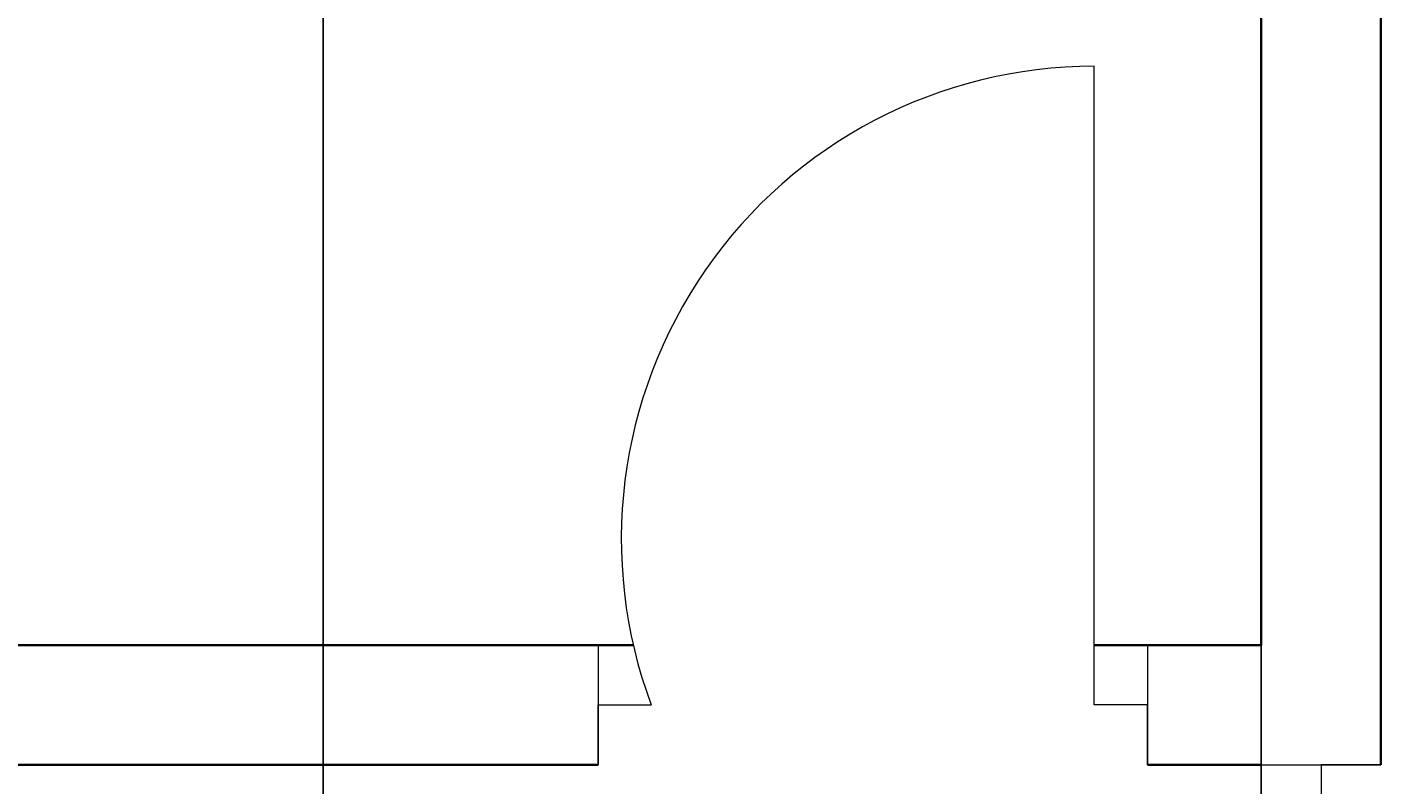
# Model space of a CAD drawing. Units: inches. Extents: x 1088 to 1703, y 668 to 1875.
# Tile 30 of 45: x 1539 to 1590, y 1539 to 1567. Entities that reach past the tile are written whole.
import ezdxf

# ---------------------------------------------------------------- set-up
doc = ezdxf.new("R2010")
doc.units = ezdxf.units.IN
for name, color, linetype, lineweight in [('A-ANNO-DIMS', 2, 'Continuous', 18), ('A-DOOR', 4, 'Continuous', 18), ('A-WALL', 7, 'Continuous', 35)]:
    doc.layers.add(name, color=color, linetype=linetype, lineweight=lineweight)
doc.styles.get("Standard").update_dxf_attribs({"font": 'arial.ttf'})
doc.dimstyles.get("Standard").update_dxf_attribs({"dimtxt": 0.18, "dimasz": 0.18, "dimexe": 0.18, "dimexo": 0.0625, "dimgap": 0.09, "dimtad": 0, "dimtih": 1, "dimtoh": 1, "dimdec": 4, "dimzin": 0, "dimdsep": 46, "dimtxsty": 'Standard', "dimcen": 0.09, "dimadec": 0, "dimazin": 0, "dimtfac": 1, "dimtdec": 4, "dimtofl": 0, "dimtmove": 0, "dimatfit": 3, "dimfxl": 1, "dimtolj": 1, "dimtzin": 0, "dimarcsym": 0})

# ---------------------------------------------------------------- blocks, each defined once
blk = doc.blocks.new('*D32')
at = {"layer": 'A-ANNO-DIMS', "color": 0, "lineweight": -2, "transparency": 16777216}
for p, q in [((1550.595, 1373.121), (1550.595, 1857.788)), ((1550.775, 1857.608), (1567.825, 1857.608)), ((1585.665, 1857.608), (1568.614, 1857.608)), ((1585.845, 1360.983), (1585.845, 1857.788))]:
    blk.add_line(p, q, dxfattribs=at)
at = {"layer": 'A-ANNO-DIMS', "color": 0, "transparency": 16777216}
for points in [[(1550.775, 1857.638), (1550.775, 1857.578), (1550.595, 1857.608)], [(1585.665, 1857.638), (1585.665, 1857.578), (1585.845, 1857.608)]]:
    blk.add_solid(points, dxfattribs=at)
at = {"layer": 'Defpoints', "color": 0, "transparency": 16777216}
for p in [(1585.845, 1857.608), (1550.595, 1373.058), (1585.845, 1360.921)]:
    blk.add_point(p, dxfattribs=at)
at = {"layer": 'A-ANNO-DIMS', "color": 0, "transparency": 16777216, "insert": (1568.22, 1857.608), "char_height": 0.18, "attachment_point": 5}
blk.add_mtext('\\A1;35.25', dxfattribs=at)

msp = doc.modelspace()

# ---------------------------------------------------------------- linework, layer by layer
at = {"layer": 'A-DOOR'}
for p, q in [((1579.571, 1541.808), (1579.571, 1565.808)), ((1560.928, 1544.058), (1560.928, 1539.558)), ((1581.571, 1544.058), (1581.571, 1539.558)), ((1560.928, 1539.558), (1560.928, 1541.808)), ((1560.928, 1541.808), (1562.928, 1541.808)), ((1581.571, 1541.808), (1579.571, 1541.808)), ((1581.571, 1539.558), (1581.571, 1541.808)), ((1585.845, 1539.558), (1590.345, 1539.558)), ((1590.345, 1539.558), (1588.095, 1539.558)), ((1588.095, 1539.558), (1588.095, 1478.749))]:
    msp.add_line(p, q, dxfattribs=at)
msp.add_arc((1579.571, 1548.037), 17.771, 90, 200.5192, dxfattribs=at)
at = {"layer": 'A-WALL'}
for p, q in [((1590.345, 1673.058), (1590.345, 1539.558)), ((1585.845, 1668.558), (1585.845, 1544.058)), ((1585.845, 1604.058), (1585.845, 1544.058)), ((1562.251, 1544.058), (1489.845, 1544.058)), ((1585.845, 1544.058), (1579.571, 1544.058)), ((1485.345, 1539.558), (1560.928, 1539.558)), ((1581.571, 1539.558), (1585.845, 1539.558))]:
    msp.add_line(p, q, dxfattribs=at)

# ---------------------------------------------------------------- dimensions: what is measured, and where the dimension line sits
at = {"layer": 'A-ANNO-DIMS'}
dim = msp.add_linear_dim(base=(1585.845, 1857.608), p1=(1550.595, 1373.058), p2=(1585.845, 1360.921), dimstyle='Standard', override={"dimdec": 2, "dimlfac": 1, "dimrnd": 0, "dimzin": 0, "dimdsep": 46, "dimlunit": 2}, dxfattribs=at)
dim.commit()
dim.dimension.update_dxf_attribs({"geometry": '*D32', "text_midpoint": (1568.22, 1857.608)})

doc.saveas('drawing.dxf')
